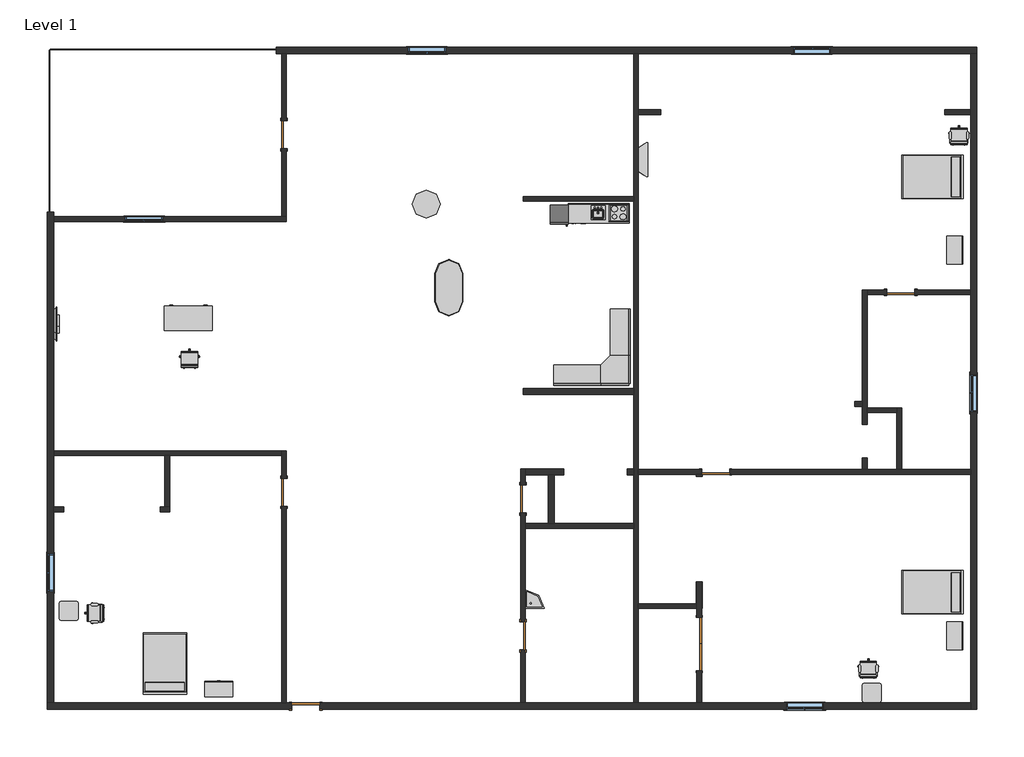
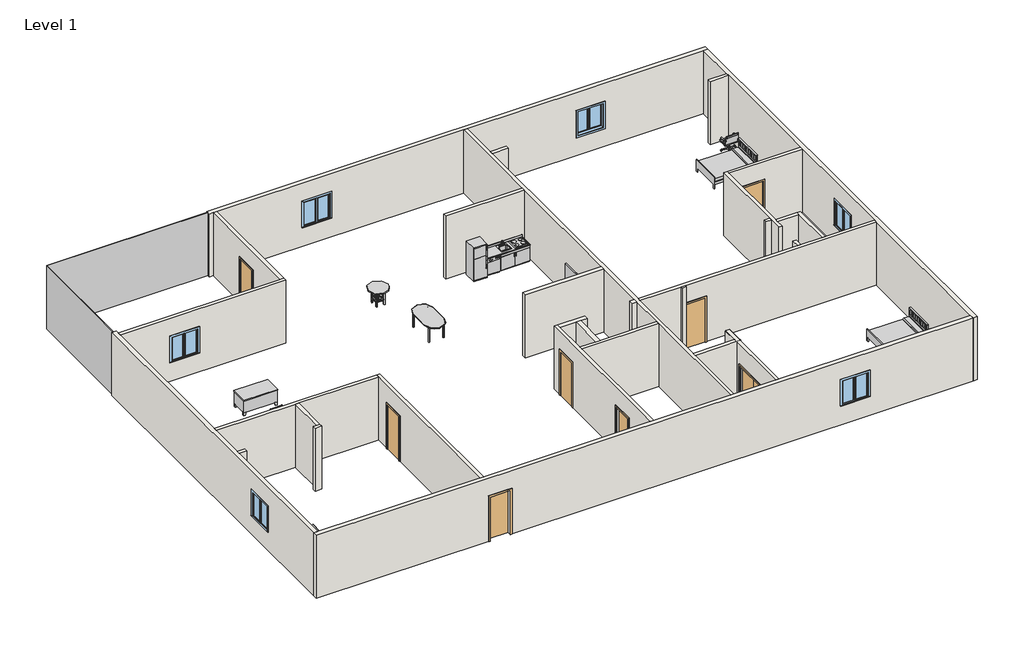
# One storey, incomplete: 32 walls, 20 furniture elements, 8 doors, 6 windows, 4 proxies, 2 flow terminals, 2 plates.
# Revit data of these elements (continued)
# Element 29 (IfcFurniture, "TV Stand : TV Stand")
#   Phase Created = New Construction
#   Materials on its faces: "Melamine - Gray", "Glass - Shelves"
# Element 30 (IfcFurniture, "Table-Dining Oval : 36\" x 72\"")
#   Phase Created = New Construction
#   Materials on its faces: "Steel, Chrome Plated", "Glass - Clear, Grey"
# Element 31 (IfcFurniture, "Table-Dining Round w Chairs : 36\" Diameter")
#   Phase Created = New Construction
#   Materials on its faces: "Pine", "Laminate, Linen, Matte"
# Elements 32, 33 (IfcFurniture, "Table-End : 24\" x 24\"")
#   Phase Created = New Construction
#   Materials on its faces: "Laminate, Ivory, Matte", "Birch"
# Element 34 (IfcFurniture, "Work Station Cubicle : 96\" x 96\"")
#   Phase Created = New Construction
#   Materials on its faces: "Textile - Light Gray", "Laminate, Ivory, Matte"
# Elements 35, 36 (IfcPlate, "System Panel : Glazed")
#   Phase Created = New Construction
#   Materials on its faces: "Glass"
# Elements 37, 38, 39, 40, 41, 42, 43, 44, 45, 46 (IfcWall, "Generic - 8\"")
#   Top Offset = 0' - 0"
#   Base Offset = 0' - 0"
#   Unconnected Height = 10' - 0"
#   wall height = 10' - 0"
#   Phase Created = New Construction
#   Base Constraint = Level 1
#   Materials on its faces: "Default Wall"
# Elements 47, 48, 49, 50, 51, 52, 53, 54, 55, 56, 57, 58, 59, 60, 61, 62, 63, 64, 65, 66, 67, 68 (IfcWall, "Generic inner wall 6\"")
#   Top Offset = 0' - 0"
#   Base Offset = 0' - 0"
#   Unconnected Height = 10' - 0"
#   wall height = 10' - 0"
#   Phase Created = New Construction
#   Base Constraint = Level 1
#   Materials on its faces: "Default Wall"
# Element 69 (IfcWindow, "Casement Dbl with Trim : 48\" x 48\"")
#   Mark = "2"
#   Phase Created = New Construction
#   Materials on its faces: "Sash", "Trim", "Glass"
# Element 70 (IfcWindow, "Casement Dbl with Trim : 48\" x 48\"")
#   Mark = "3"
#   Phase Created = New Construction
#   Materials on its faces: "Sash", "Trim", "Glass"
# Element 71 (IfcWindow, "Casement Dbl with Trim : 48\" x 48\"")
#   Mark = "4"
#   Phase Created = New Construction
#   Materials on its faces: "Sash", "Trim", "Glass"
# Element 72 (IfcWindow, "Casement Dbl with Trim : 48\" x 48\"")
#   Mark = "5"
#   Phase Created = New Construction
#   Materials on its faces: "Sash", "Trim", "Glass"
# Element 73 (IfcWindow, "Casement Dbl with Trim : 48\" x 48\"")
#   Mark = "6"
#   Phase Created = New Construction
#   Materials on its faces: "Sash", "Trim", "Glass"
# Element 74 (IfcWindow, "Casement Dbl with Trim : 48\" x 48\"")
#   Mark = "1"
#   Phase Created = New Construction
#   Materials on its faces: "Sash", "Trim", "Glass"
# Materials
#   "Steel, Chrome Plated": class "Metal", colour RGB 17 17 17, transparency 0, Description = "Chromiuim plated steel", Cost = 0
#   "Steel, Polished": class "Metal", colour RGB 57 57 57, transparency 0, Description = "Polished steel", Cost = 0
#   "Steel, Paint Finish, Ivory, Glossy": class "Metal", colour RGB 247 247 239, transparency 0, Description = "Steel, paint finish, ivory, glossy", Cost = 0
#   "Plastic, Opaque Black": class "Plastic", colour RGB 0 0 0, transparency 0.7, Description = "Plastic, generic, opaque black", Cost = 0
#   "Cabinets": colour RGB 249 249 249, transparency 0
#   "Cabinets - Handles": class "Metal", colour RGB 57 57 57, transparency 0
#   "Wood - Birch - Solid Stained Light Low Gloss": class "Wood", colour RGB 210 159 95, transparency 0, Cost = 0
#   "Paint - Sienna": colour RGB 118 70 51, transparency 0, Cost = 0
#   "Door - Panel": class "Wood", colour RGB 210 159 95, transparency 0
#   "Door - Frame": colour RGB 118 70 51, transparency 0
#   "Birch": class "Wood", colour RGB 224 178 126, transparency 0, Description = "Betula Alleghaniensis", Cost = 0
#   "Linen, White": class "Textile", colour RGB 247 247 239, transparency 0, Description = "Linen, white", Cost = 0
#   "Textile - Slate Blue": class "Fabric", colour RGB 98 102 118, transparency 0
#   "Laminate, Ivory, Matte": class "Plastic", colour RGB 247 247 239, transparency 0, Description = "Plastic Laminate - Ivory, Matte", Cost = 0
#   "Cherry": class "Wood", colour RGB 226 177 128, transparency 0, Description = "Prunus Serotina", Cost = 0
#   "Melamine - Gray": class "Wood", colour RGB 49 49 49, transparency 0
#   "Glass - Clear, Grey": class "Glass", colour RGB 252 255 255, transparency 0.64
#   "Pine": class "Wood", colour RGB 223 192 134, transparency 0, Description = "Pinus Echinata", Cost = 0
#   "Laminate, Linen, Matte": class "Plastic", colour RGB 249 239 230, transparency 0, Description = "Plastic Laminate - Linen, Matte", Cost = 0
#   "Textile - Light Gray": class "Fabric", colour RGB 204 204 204, transparency 0
#   "Glass": class "Glass", colour RGB 0 128 192, transparency 0.75, Description = "Soda Lime Glass", Cost = 0
#   "Sash": class "Wood", colour RGB 224 178 126, transparency 0
#   "Trim": class "Wood", colour RGB 224 178 126, transparency 0
#   "Counter Top": class "Wood", colour RGB 226 177 128, transparency 0
#   "TV - Black": colour RGB 49 49 49, transparency 0
#   "TV - Glass": colour RGB 157 157 157, transparency 0.9
#   "TV - Screen": colour RGB 0 0 0, transparency 0
#   "Glass - Shelves": class "Glass", colour RGB 167 167 167, transparency 0.9
#   "Default Wall": colour RGB 128 128 128, transparency 0
